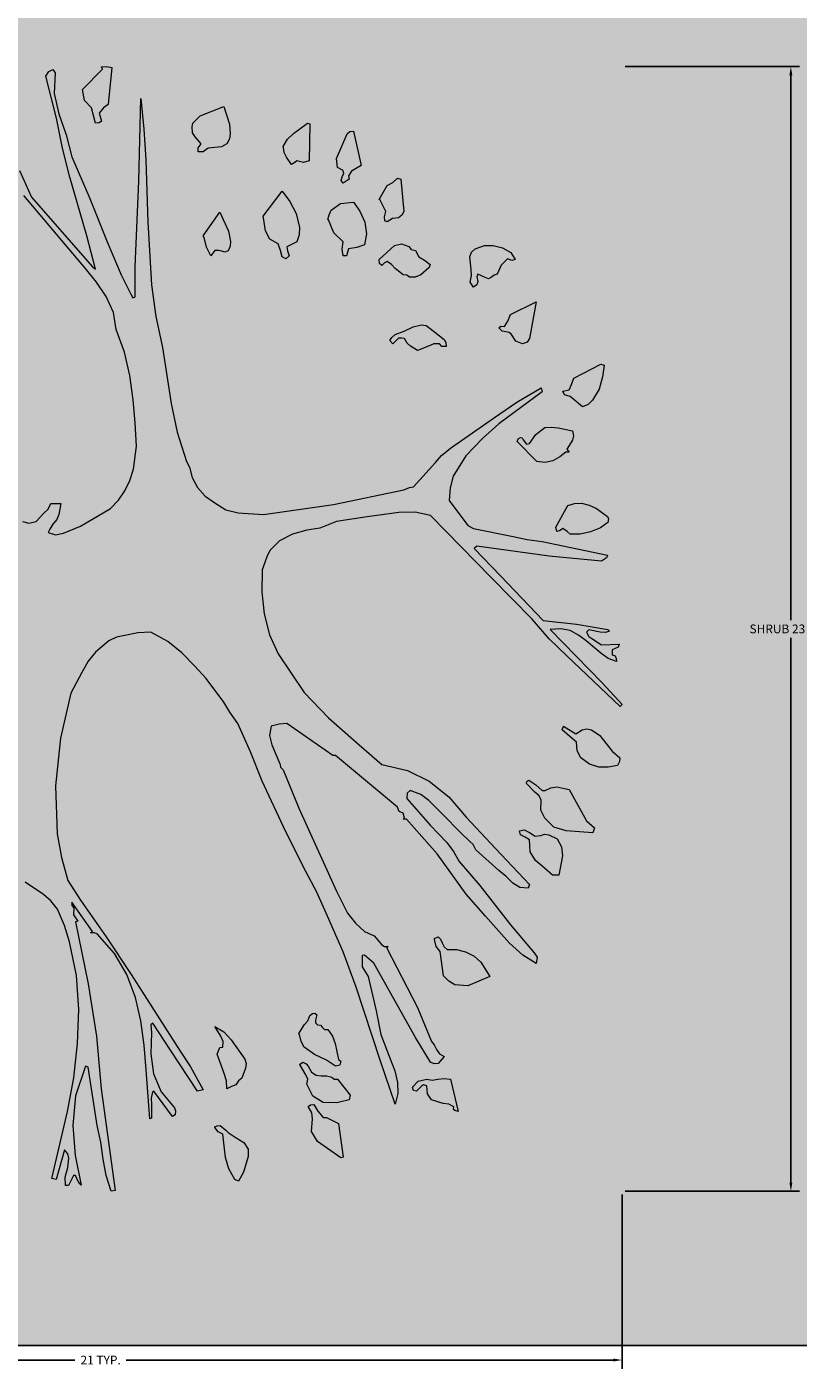
# Model space of a CAD drawing. Units: inches. Extents: x 84 to 1044, y -280 to 906.
# Tile 19 of 105: x 684 to 700, y -113 to -86. Entities that reach past the tile are written whole.
import ezdxf

# ---------------------------------------------------------------- set-up
doc = ezdxf.new("R2010")
doc.units = ezdxf.units.IN
for name, color, linetype, lineweight in [('A-ANNO-DIMS', 2, 'Continuous', 18), ('C-PROP', 7, 'Continuous', 25), ('L-PLNT', 114, 'Continuous', 15)]:
    doc.layers.add(name, color=color, linetype=linetype, lineweight=lineweight)
doc.layers.add('L-PLNT-PATT', color=9, linetype='Continuous', lineweight=9, true_color=0xafd9aa)
doc.styles.get("Standard").update_dxf_attribs({"font": 'arial.ttf'})
doc.dimstyles.get("Standard").update_dxf_attribs({"dimtxt": 0.18, "dimasz": 0.18, "dimexe": 0.18, "dimexo": 0.0625, "dimgap": 0.09, "dimtad": 0, "dimtih": 1, "dimtoh": 1, "dimdec": 4, "dimzin": 0, "dimdsep": 46, "dimtxsty": 'Standard', "dimcen": 0.09, "dimadec": 0, "dimazin": 0, "dimtfac": 1, "dimtdec": 4, "dimtofl": 0, "dimtmove": 0, "dimatfit": 3, "dimfxl": 1, "dimtolj": 1, "dimtzin": 0, "dimarcsym": 0})

# ---------------------------------------------------------------- blocks, each defined once
blk = doc.blocks.new('A$C37E508DF')
for p, q in [((0.6329, 1.5111), (0.6367, 1.5175)), ((0.6367, 1.5175), (0.6423, 1.5201)), ((0.6423, 1.5201), (0.6453, 1.5158)), ((0.6453, 1.5158), (0.644, 1.4879)), ((0.6826, 1.493), (0.7096, 1.5209)), ((0.7083, 1.5239), (0.7152, 1.5244)), ((0.7096, 1.5209), (0.7083, 1.5239)), ((0.7152, 1.5244), (0.7225, 1.5231)), ((0.7225, 1.5231), (0.7174, 1.4729)), ((0.6475, 1.4545), (0.6329, 1.5111)), ((0.644, 1.4879), (0.6505, 1.46)), ((0.6852, 1.4785), (0.6826, 1.493)), ((0.6946, 1.4682), (0.6852, 1.4785)), ((0.7589, 1.3691), (0.7615, 1.481)), ((0.7615, 1.481), (0.7658, 1.4395)), ((0.6505, 1.46), (0.6603, 1.4317)), ((0.6976, 1.4579), (0.6946, 1.4682)), ((0.7109, 1.4682), (0.7053, 1.4609)), ((0.7053, 1.4609), (0.7083, 1.4502)), ((0.7174, 1.4729), (0.7109, 1.4682)), ((0.8421, 1.4575), (0.8739, 1.4703)), ((0.8739, 1.4703), (0.882, 1.4463)), ((0.6552, 1.4137), (0.6475, 1.4545)), ((0.7002, 1.4476), (0.6976, 1.4579)), ((0.7049, 1.448), (0.7002, 1.4476)), ((0.7083, 1.4502), (0.7049, 1.448)), ((0.831, 1.4424), (0.8323, 1.4476)), ((0.8318, 1.4343), (0.831, 1.4424)), ((0.8323, 1.4476), (0.8357, 1.451)), ((0.8357, 1.451), (0.8421, 1.4575)), ((0.882, 1.4463), (0.8829, 1.433)), ((0.9686, 1.4334), (0.9875, 1.4476)), ((0.9875, 1.4476), (0.9905, 1.4467)), ((0.9905, 1.4467), (0.9896, 1.3966)), ((0.6603, 1.4317), (0.668, 1.4021)), ((0.7658, 1.4395), (0.7684, 1.3979)), ((0.8353, 1.4292), (0.8318, 1.4343)), ((0.8434, 1.4197), (0.8353, 1.4292)), ((0.8816, 1.4262), (0.8781, 1.4197)), ((0.8829, 1.433), (0.8816, 1.4262)), ((0.9545, 1.4159), (0.9605, 1.4257)), ((0.9605, 1.4257), (0.9686, 1.4334)), ((1.0269, 1.3996), (1.0411, 1.433)), ((1.0411, 1.433), (1.045, 1.4365)), ((1.045, 1.4365), (1.0497, 1.4369)), ((1.0497, 1.4369), (1.0604, 1.3901)), ((0.6655, 1.3743), (0.6552, 1.4137)), ((0.8391, 1.4141), (0.8434, 1.4197)), ((0.8395, 1.4086), (0.8391, 1.4141)), ((0.846, 1.4086), (0.8395, 1.4086)), ((0.8528, 1.4137), (0.846, 1.4086)), ((0.8619, 1.4146), (0.8528, 1.4137)), ((0.8709, 1.4154), (0.8619, 1.4146)), ((0.8781, 1.4197), (0.8709, 1.4154)), ((0.9549, 1.4146), (0.9545, 1.4159)), ((0.9558, 1.4077), (0.9549, 1.4146)), ((0.9592, 1.4017), (0.9558, 1.4077)), ((0.668, 1.4021), (0.6925, 1.3455)), ((0.7684, 1.3979), (0.771, 1.3134)), ((0.966, 1.3914), (0.9592, 1.4017)), ((0.9703, 1.3944), (0.966, 1.3914)), ((0.9733, 1.3966), (0.9703, 1.3944)), ((0.9819, 1.3944), (0.9733, 1.3966)), ((0.9896, 1.3966), (0.9819, 1.3944)), ((1.0282, 1.3876), (1.0269, 1.3996)), ((1.0359, 1.3833), (1.0282, 1.3876)), ((1.0604, 1.3901), (1.0471, 1.3824)), ((0.5969, 1.3833), (0.6132, 1.3472)), ((0.6882, 1.2949), (0.6655, 1.3743)), ((0.7538, 1.2529), (0.7589, 1.3691)), ((1.0334, 1.37), (1.0351, 1.376)), ((1.0359, 1.3661), (1.0334, 1.37)), ((1.0351, 1.376), (1.0368, 1.3794)), ((1.0368, 1.3794), (1.0359, 1.3833)), ((1.0441, 1.3717), (1.0359, 1.3661)), ((1.0471, 1.3824), (1.0432, 1.3764)), ((1.0432, 1.3764), (1.0441, 1.3717)), ((1.1033, 1.367), (1.1097, 1.373)), ((1.1097, 1.373), (1.114, 1.3717)), ((1.114, 1.3717), (1.1183, 1.328)), ((0.9274, 1.3215), (0.9532, 1.3554)), ((0.9532, 1.3554), (0.9635, 1.3413)), ((1.0848, 1.3443), (1.0955, 1.3631)), ((1.0955, 1.3631), (1.1033, 1.367)), ((0.6595, 1.2829), (0.6029, 1.3494)), ((0.6132, 1.3472), (0.6959, 1.2529)), ((0.6925, 1.3455), (0.7161, 1.2868)), ((0.9635, 1.3413), (0.9721, 1.325)), ((1.0197, 1.3297), (1.0321, 1.3387)), ((1.0321, 1.3387), (1.0497, 1.3404)), ((1.0497, 1.3404), (1.0587, 1.3284)), ((1.0861, 1.343), (1.0848, 1.3443)), ((1.0938, 1.328), (1.0861, 1.343)), ((0.846, 1.2949), (0.8687, 1.3271)), ((0.8687, 1.3271), (0.8803, 1.3014)), ((0.9279, 1.3194), (0.9274, 1.3215)), ((0.9305, 1.3018), (0.9279, 1.3194)), ((0.9721, 1.325), (0.9768, 1.3061)), ((1.0149, 1.3172), (1.0171, 1.3232)), ((1.0162, 1.3164), (1.0149, 1.3172)), ((1.0231, 1.2988), (1.0162, 1.3164)), ((1.0171, 1.3232), (1.0197, 1.3297)), ((1.0587, 1.3284), (1.0651, 1.3134)), ((1.0917, 1.3207), (1.0938, 1.328)), ((1.0925, 1.3151), (1.0917, 1.3207)), ((1.0955, 1.3138), (1.0925, 1.3151)), ((1.1028, 1.3185), (1.0955, 1.3138)), ((1.111, 1.3194), (1.1028, 1.3185)), ((1.1153, 1.3228), (1.111, 1.3194)), ((1.1183, 1.328), (1.1153, 1.3228)), ((0.771, 1.3134), (0.7761, 1.2285)), ((0.8803, 1.3014), (0.8833, 1.2872)), ((0.9365, 1.2902), (0.9305, 1.3018)), ((0.9763, 1.2962), (0.9733, 1.2868)), ((0.9768, 1.3061), (0.9763, 1.2962)), ((1.0359, 1.2868), (1.0231, 1.2988)), ((1.0677, 1.2975), (1.0647, 1.2829)), ((1.0651, 1.3134), (1.0677, 1.2975)), ((0.6865, 1.2508), (0.6595, 1.2829)), ((0.7002, 1.2495), (0.6882, 1.2949)), ((0.7161, 1.2868), (0.7349, 1.2422)), ((0.8473, 1.2924), (0.846, 1.2949)), ((0.8507, 1.2795), (0.8473, 1.2924)), ((0.8567, 1.2679), (0.8507, 1.2795)), ((0.8829, 1.2808), (0.8799, 1.2744)), ((0.8833, 1.2872), (0.8829, 1.2808)), ((0.9476, 1.2842), (0.9365, 1.2902)), ((0.951, 1.2748), (0.9476, 1.2842)), ((0.9733, 1.2868), (0.9596, 1.2799)), ((0.9596, 1.2799), (0.9605, 1.2744)), ((1.0347, 1.2769), (1.0359, 1.2868)), ((1.0432, 1.2774), (1.0402, 1.2679)), ((1.0544, 1.2791), (1.0432, 1.2774)), ((1.0647, 1.2829), (1.0544, 1.2791)), ((1.0848, 1.2628), (1.1054, 1.2817)), ((1.1054, 1.2817), (1.1148, 1.2842)), ((1.1148, 1.2842), (1.1247, 1.2804)), ((1.1247, 1.2804), (1.1281, 1.2765)), ((1.21, 1.2726), (1.2147, 1.2774)), ((1.2147, 1.2774), (1.2276, 1.2817)), ((1.2276, 1.2817), (1.2392, 1.2817)), ((1.2392, 1.2817), (1.2521, 1.2787)), ((1.2521, 1.2787), (1.2632, 1.2722)), ((0.8619, 1.2752), (0.8567, 1.2679)), ((0.867, 1.2752), (0.8619, 1.2752)), ((0.8713, 1.2739), (0.867, 1.2752)), ((0.8756, 1.2726), (0.8713, 1.2739)), ((0.8799, 1.2744), (0.8756, 1.2726)), ((0.9532, 1.2666), (0.951, 1.2748)), ((0.9583, 1.2636), (0.9532, 1.2666)), ((0.9626, 1.2679), (0.9583, 1.2636)), ((0.9605, 1.2744), (0.9626, 1.2679)), ((1.0359, 1.2679), (1.0347, 1.2769)), ((1.0402, 1.2679), (1.0359, 1.2679)), ((1.0852, 1.2576), (1.0848, 1.2628)), ((1.0955, 1.2602), (1.0921, 1.2585)), ((1.1015, 1.2559), (1.0955, 1.2602)), ((1.1281, 1.2765), (1.1341, 1.2752)), ((1.1341, 1.2752), (1.1384, 1.2666)), ((1.1384, 1.2666), (1.1461, 1.2619)), ((1.1461, 1.2619), (1.1539, 1.2559)), ((1.2075, 1.2666), (1.21, 1.2726)), ((1.2096, 1.2491), (1.2075, 1.2666)), ((1.2585, 1.2636), (1.2503, 1.2551)), ((1.2645, 1.2615), (1.2585, 1.2636)), ((1.2632, 1.2722), (1.2692, 1.2628)), ((1.2692, 1.2628), (1.2645, 1.2615)), ((0.7015, 1.2323), (0.6865, 1.2508)), ((0.6959, 1.2529), (0.7002, 1.2495)), ((0.7349, 1.2422), (0.7482, 1.216)), ((0.7538, 1.2122), (0.7538, 1.2529)), ((1.0883, 1.2546), (1.0852, 1.2576)), ((1.0921, 1.2585), (1.0883, 1.2546)), ((1.1063, 1.2508), (1.1015, 1.2559)), ((1.117, 1.2422), (1.1063, 1.2508)), ((1.1221, 1.2418), (1.117, 1.2422)), ((1.126, 1.2388), (1.1221, 1.2418)), ((1.141, 1.2422), (1.1337, 1.2388)), ((1.1526, 1.2521), (1.141, 1.2422)), ((1.1539, 1.2559), (1.1526, 1.2521)), ((1.2079, 1.2323), (1.21, 1.2409)), ((1.21, 1.2409), (1.2096, 1.2491)), ((1.2186, 1.2431), (1.2173, 1.2392)), ((1.2285, 1.2383), (1.2186, 1.2431)), ((1.2405, 1.2418), (1.2371, 1.2388)), ((1.2448, 1.2431), (1.2405, 1.2418)), ((1.2503, 1.2551), (1.2448, 1.2431)), ((0.7148, 1.2126), (0.7015, 1.2323)), ((0.7761, 1.2285), (0.7821, 1.1856)), ((1.1337, 1.2388), (1.126, 1.2388)), ((1.2126, 1.2251), (1.2079, 1.2323)), ((1.2169, 1.2285), (1.2126, 1.2251)), ((1.2186, 1.2332), (1.2169, 1.2285)), ((1.2173, 1.2392), (1.2186, 1.2332)), ((1.2328, 1.2366), (1.2285, 1.2383)), ((1.2371, 1.2388), (1.2328, 1.2366)), ((0.7246, 1.1908), (0.7148, 1.2126)), ((0.7482, 1.216), (0.7508, 1.2109)), ((0.7508, 1.2109), (0.7538, 1.2122)), ((1.2628, 1.1882), (1.2975, 1.2053)), ((1.2975, 1.2053), (1.2885, 1.1556)), ((0.7281, 1.168), (0.7246, 1.1908)), ((1.2589, 1.1792), (1.2628, 1.1882)), ((0.7396, 1.1371), (0.7281, 1.168)), ((0.7821, 1.1856), (0.7911, 1.1436)), ((1.1187, 1.1655), (1.1307, 1.1714)), ((1.1307, 1.1714), (1.1423, 1.1744)), ((1.1423, 1.1744), (1.1483, 1.1732)), ((1.1483, 1.1732), (1.1539, 1.1693)), ((1.1539, 1.1693), (1.1727, 1.1543)), ((1.2469, 1.1702), (1.2495, 1.1723)), ((1.2478, 1.1693), (1.2469, 1.1702)), ((1.2516, 1.1659), (1.2478, 1.1693)), ((1.2495, 1.1723), (1.2546, 1.1719)), ((1.2546, 1.1719), (1.2589, 1.1792)), ((1.099, 1.153), (1.102, 1.1573)), ((1.1033, 1.1487), (1.099, 1.153)), ((1.102, 1.1573), (1.1063, 1.1612)), ((1.111, 1.156), (1.1033, 1.1487)), ((1.1063, 1.1612), (1.1187, 1.1655)), ((1.1153, 1.1564), (1.111, 1.156)), ((1.1191, 1.1556), (1.1153, 1.1564)), ((1.1226, 1.1492), (1.1191, 1.1556)), ((1.1727, 1.1543), (1.1749, 1.1504)), ((1.1749, 1.1504), (1.1757, 1.1449)), ((1.2563, 1.1646), (1.2516, 1.1659)), ((1.2611, 1.1637), (1.2563, 1.1646)), ((1.2641, 1.1612), (1.2611, 1.1637)), ((1.2701, 1.1522), (1.2641, 1.1612)), ((1.2791, 1.1487), (1.2701, 1.1522)), ((1.2851, 1.1509), (1.2791, 1.1487)), ((1.2885, 1.1556), (1.2851, 1.1509)), ((0.7469, 1.1054), (0.7396, 1.1371)), ((0.7911, 1.1436), (0.8027, 1.0677)), ((1.1273, 1.1453), (1.1226, 1.1492)), ((1.1367, 1.1393), (1.1273, 1.1453)), ((1.1517, 1.1453), (1.1367, 1.1393)), ((1.1586, 1.1483), (1.1517, 1.1453)), ((1.1663, 1.1487), (1.1586, 1.1483)), ((1.1697, 1.1449), (1.1663, 1.1487)), ((1.1757, 1.1449), (1.1697, 1.1449)), ((1.3485, 1.102), (1.385, 1.1209)), ((1.385, 1.1209), (1.3897, 1.1196)), ((1.3897, 1.1196), (1.3875, 1.1037)), ((0.7512, 1.0728), (0.7469, 1.1054)), ((1.3455, 1.0934), (1.3485, 1.102)), ((1.3875, 1.1037), (1.3828, 1.087)), ((1.3057, 1.0835), (1.2469, 1.0402)), ((1.2713, 1.0694), (1.3044, 1.0887)), ((1.3044, 1.0887), (1.3057, 1.0835)), ((1.3335, 1.0844), (1.3421, 1.0861)), ((1.3361, 1.0793), (1.3335, 1.0844)), ((1.3434, 1.0771), (1.3361, 1.0793)), ((1.3421, 1.0861), (1.3455, 1.0934)), ((1.349, 1.0728), (1.3434, 1.0771)), ((1.3828, 1.087), (1.3738, 1.072)), ((0.7538, 1.0415), (0.7512, 1.0728)), ((0.8027, 1.0677), (0.8108, 1.0287)), ((1.2409, 1.0488), (1.2713, 1.0694)), ((1.3605, 1.063), (1.349, 1.0728)), ((1.3678, 1.0664), (1.3605, 1.063)), ((1.3738, 1.072), (1.3678, 1.0664)), ((0.7559, 1.0098), (0.7538, 1.0415)), ((1.1813, 1.0072), (1.2409, 1.0488)), ((1.2469, 1.0402), (1.2246, 1.0201)), ((0.8108, 1.0287), (0.8233, 0.9892)), ((1.2731, 1.0197), (1.2761, 1.0218)), ((1.2761, 1.0218), (1.2786, 1.0209)), ((1.2885, 1.0136), (1.2971, 1.0257)), ((1.2971, 1.0257), (1.3091, 1.0351)), ((1.3091, 1.0351), (1.3185, 1.0355)), ((1.3185, 1.0355), (1.3275, 1.0347)), ((1.3275, 1.0347), (1.3468, 1.0308)), ((1.3468, 1.0308), (1.3481, 1.0239)), ((1.3481, 1.0239), (1.3468, 1.018)), ((0.7516, 0.9785), (0.7559, 1.0098)), ((1.1693, 0.9974), (1.1813, 1.0072)), ((1.2246, 1.0201), (1.2023, 0.9969)), ((1.2718, 1.0162), (1.2731, 1.0197)), ((1.2984, 0.9892), (1.2718, 1.0162)), ((1.2786, 1.0209), (1.2799, 1.0184)), ((1.2799, 1.0184), (1.2842, 1.0124)), ((1.2842, 1.0124), (1.2885, 1.0136)), ((1.3468, 1.018), (1.3391, 1.0059)), ((1.3391, 1.0059), (1.3421, 1.0016)), ((0.8233, 0.9892), (0.8275, 0.9815)), ((1.1311, 0.9549), (1.1612, 0.9879)), ((1.1612, 0.9879), (1.1693, 0.9974)), ((1.2023, 0.9969), (1.1852, 0.9691)), ((1.3095, 0.9875), (1.2984, 0.9892)), ((1.3202, 0.9901), (1.3095, 0.9875)), ((1.3297, 0.9952), (1.3202, 0.9901)), ((1.3378, 1.0016), (1.3297, 0.9952)), ((1.3421, 1.0016), (1.3378, 1.0016)), ((0.7469, 0.9635), (0.7516, 0.9785)), ((0.8275, 0.9815), (0.8314, 0.9673)), ((0.8314, 0.9673), (0.8383, 0.954)), ((1.1852, 0.9691), (1.1809, 0.9532)), ((0.7315, 0.9365), (0.7401, 0.9493)), ((0.7401, 0.9493), (0.7469, 0.9635)), ((0.8383, 0.954), (0.8486, 0.942)), ((1.0227, 0.9309), (1.1183, 0.9506)), ((1.1183, 0.9506), (1.1256, 0.954)), ((1.1256, 0.954), (1.1311, 0.9549)), ((1.1809, 0.9532), (1.1796, 0.936)), ((0.6359, 0.9245), (0.6397, 0.9322)), ((0.6397, 0.9322), (0.653, 0.9322)), ((0.653, 0.9322), (0.6505, 0.9172)), ((0.7203, 0.9253), (0.7315, 0.9365)), ((0.8486, 0.942), (0.8619, 0.933)), ((0.8619, 0.933), (0.8769, 0.9236)), ((0.9279, 0.9172), (1.0227, 0.9309)), ((1.1796, 0.936), (1.2049, 0.9022)), ((1.3404, 0.9292), (1.3494, 0.9322)), ((1.3494, 0.9322), (1.3592, 0.9326)), ((1.3592, 0.9326), (1.3695, 0.93)), ((0.6196, 0.9077), (0.6303, 0.9189)), ((0.6303, 0.9189), (0.6359, 0.9245)), ((0.6505, 0.9172), (0.6479, 0.9103)), ((0.6796, 0.9013), (0.7203, 0.9253)), ((0.8769, 0.9236), (0.8936, 0.9193)), ((0.8936, 0.9193), (0.9279, 0.9172)), ((1.0685, 0.9142), (1.0269, 0.9077)), ((1.1114, 0.9198), (1.0685, 0.9142)), ((1.1333, 0.9202), (1.1114, 0.9198)), ((1.1543, 0.9159), (1.1333, 0.9202)), ((1.2371, 0.8314), (1.1543, 0.9159)), ((1.3241, 0.9), (1.3404, 0.9292)), ((1.3695, 0.93), (1.3794, 0.9253)), ((1.3794, 0.9253), (1.394, 0.9146)), ((1.394, 0.9146), (1.3957, 0.9112)), ((0.6011, 0.9077), (0.6097, 0.9056)), ((0.6097, 0.9056), (0.6196, 0.9077)), ((0.6384, 0.8974), (0.6359, 0.8927)), ((0.6423, 0.9039), (0.6384, 0.8974)), ((0.6479, 0.9103), (0.6423, 0.9039)), ((0.6569, 0.8919), (0.6796, 0.9013)), ((0.9866, 0.8962), (0.9673, 0.8906)), ((1.0042, 0.8987), (0.9866, 0.8962)), ((1.0269, 0.9077), (1.0042, 0.8987)), ((1.2049, 0.9022), (1.2126, 0.8983)), ((1.2126, 0.8983), (1.2662, 0.8876)), ((1.3254, 0.8944), (1.3241, 0.9)), ((1.3301, 0.8957), (1.3254, 0.8944)), ((1.3335, 0.8983), (1.3301, 0.8957)), ((1.3395, 0.8944), (1.3335, 0.8983)), ((1.3434, 0.8906), (1.3395, 0.8944)), ((1.3846, 0.8992), (1.3713, 0.8936)), ((1.3948, 0.9065), (1.3846, 0.8992)), ((1.3957, 0.9112), (1.3948, 0.9065)), ((0.6359, 0.8927), (0.6457, 0.8897)), ((0.6457, 0.8897), (0.6569, 0.8919)), ((0.9498, 0.8816), (0.9369, 0.8687)), ((0.9673, 0.8906), (0.9498, 0.8816)), ((1.2662, 0.8876), (1.2855, 0.8833)), ((1.2855, 0.8833), (1.3057, 0.8807)), ((1.3057, 0.8807), (1.394, 0.8623)), ((1.3571, 0.8906), (1.3434, 0.8906)), ((1.3713, 0.8936), (1.3571, 0.8906)), ((0.933, 0.861), (0.9296, 0.852)), ((0.9369, 0.8687), (0.933, 0.861)), ((1.2169, 0.8743), (1.2135, 0.8713)), ((1.2135, 0.8713), (1.2491, 0.834)), ((1.3151, 0.8606), (1.2169, 0.8743)), ((1.3863, 0.8541), (1.3151, 0.8606)), ((1.3927, 0.8584), (1.3863, 0.8541)), ((1.394, 0.8623), (1.3927, 0.8584)), ((0.9262, 0.8421), (0.9257, 0.8121)), ((0.9296, 0.852), (0.9262, 0.8421)), ((1.2919, 0.7752), (1.2371, 0.8314)), ((1.2491, 0.834), (1.3069, 0.7735)), ((0.9257, 0.8121), (0.9287, 0.7825)), ((0.9287, 0.7825), (0.936, 0.7542)), ((1.3151, 0.7487), (1.2919, 0.7752)), ((1.3069, 0.7735), (1.352, 0.7684)), ((1.352, 0.7684), (1.3948, 0.7615)), ((0.7285, 0.7512), (0.7182, 0.7461)), ((0.7401, 0.7534), (0.7285, 0.7512)), ((0.7577, 0.7568), (0.7401, 0.7534)), ((0.7752, 0.7577), (0.7577, 0.7568)), ((0.798, 0.7452), (0.7752, 0.7577)), ((0.936, 0.7542), (0.9476, 0.7285)), ((1.3391, 0.7255), (1.3151, 0.7487)), ((1.3309, 0.7624), (1.3164, 0.7615)), ((1.3164, 0.7615), (1.3871, 0.6891)), ((1.3434, 0.7598), (1.3309, 0.7624)), ((1.355, 0.7538), (1.3434, 0.7598)), ((1.3653, 0.7461), (1.355, 0.7538)), ((1.3687, 0.7607), (1.3657, 0.7577)), ((1.3657, 0.7577), (1.3691, 0.7521)), ((1.3841, 0.7577), (1.3687, 0.7607)), ((1.3691, 0.7521), (1.3743, 0.7482)), ((1.3743, 0.7482), (1.3863, 0.7405)), ((1.3914, 0.7572), (1.3841, 0.7577)), ((1.397, 0.759), (1.3914, 0.7572)), ((1.3948, 0.7615), (1.397, 0.759)), ((0.7002, 0.7307), (0.6903, 0.7186)), ((0.7182, 0.7461), (0.7002, 0.7307)), ((0.8173, 0.7298), (0.798, 0.7452)), ((0.8344, 0.7122), (0.8173, 0.7298)), ((1.3854, 0.7294), (1.3653, 0.7461)), ((1.3863, 0.7405), (1.4099, 0.7414)), ((1.4086, 0.7375), (1.4004, 0.7337)), ((1.4004, 0.7337), (1.4004, 0.7272)), ((1.4099, 0.7414), (1.4086, 0.7375)), ((0.6903, 0.7186), (0.6818, 0.7032)), ((0.8503, 0.6951), (0.8344, 0.7122)), ((0.9476, 0.7285), (0.9828, 0.6762)), ((1.4116, 0.6569), (1.3391, 0.7255)), ((1.3953, 0.7221), (1.3854, 0.7294)), ((1.4064, 0.7178), (1.3953, 0.7221)), ((1.4004, 0.7272), (1.4047, 0.7255)), ((1.4047, 0.7255), (1.406, 0.7221)), ((1.406, 0.7221), (1.4064, 0.7178)), ((0.6818, 0.7032), (0.6667, 0.6749)), ((0.8739, 0.6629), (0.8503, 0.6951)), ((0.9828, 0.6762), (1.0162, 0.6415)), ((1.3871, 0.6891), (1.4141, 0.6599)), ((0.6667, 0.6749), (0.6526, 0.614)), ((0.8824, 0.6492), (0.8739, 0.6629)), ((1.4141, 0.6599), (1.4116, 0.6569)), ((0.8932, 0.6342), (0.8824, 0.6492)), ((1.0162, 0.6415), (1.0574, 0.605)), ((0.9103, 0.5956), (0.8932, 0.6342)), ((0.9382, 0.6303), (0.936, 0.6179)), ((0.9493, 0.6333), (0.9382, 0.6303)), ((0.9596, 0.6342), (0.9493, 0.6333)), ((1.0218, 0.5904), (0.9596, 0.6342)), ((1.3327, 0.6252), (1.3348, 0.6303)), ((1.343, 0.6162), (1.3327, 0.6252)), ((1.3348, 0.6303), (1.3511, 0.62)), ((1.3511, 0.62), (1.3601, 0.6256)), ((1.3601, 0.6256), (1.3661, 0.6269)), ((1.3661, 0.6269), (1.3725, 0.6252)), ((1.3725, 0.6252), (1.3837, 0.6175)), ((0.6526, 0.614), (0.6457, 0.5497)), ((0.936, 0.6179), (0.939, 0.605)), ((0.939, 0.605), (0.9506, 0.5784)), ((1.0574, 0.605), (1.0883, 0.5784)), ((1.352, 0.6089), (1.343, 0.6162)), ((1.3533, 0.5969), (1.352, 0.6089)), ((1.3837, 0.6175), (1.3918, 0.6072)), ((1.3918, 0.6072), (1.4004, 0.5964)), ((0.9262, 0.5557), (0.9103, 0.5956)), ((1.0256, 0.5904), (1.0218, 0.5904)), ((1.1097, 0.5205), (1.0256, 0.5904)), ((1.358, 0.5874), (1.3533, 0.5969)), ((1.37, 0.5789), (1.358, 0.5874)), ((1.4004, 0.5964), (1.4111, 0.5874)), ((1.4111, 0.5874), (1.4103, 0.5823)), ((0.9506, 0.5784), (0.951, 0.5746)), ((0.951, 0.5746), (0.9545, 0.5711)), ((0.9545, 0.5711), (0.9759, 0.5193)), ((1.0883, 0.5784), (1.123, 0.5703)), ((1.123, 0.5703), (1.1526, 0.5557)), ((1.3824, 0.575), (1.37, 0.5789)), ((1.3953, 0.5746), (1.3824, 0.575)), ((1.4077, 0.5771), (1.3953, 0.5746)), ((1.4103, 0.5823), (1.4077, 0.5771)), ((0.6457, 0.5497), (0.6483, 0.4845)), ((0.9583, 0.4871), (0.9262, 0.5557)), ((1.1526, 0.5557), (1.1792, 0.5347)), ((1.2842, 0.554), (1.2855, 0.5557)), ((1.2842, 0.5527), (1.2842, 0.554)), ((1.2958, 0.5407), (1.2842, 0.5527)), ((1.2855, 0.5557), (1.2876, 0.557)), ((1.2876, 0.557), (1.2971, 0.551)), ((1.2971, 0.551), (1.3057, 0.5433)), ((1.3172, 0.5467), (1.3254, 0.548)), ((1.3254, 0.548), (1.3421, 0.5446)), ((1.1226, 0.5394), (1.1221, 0.5325)), ((1.1221, 0.5325), (1.1539, 0.4961)), ((1.1268, 0.5433), (1.1226, 0.5394)), ((1.141, 0.5377), (1.1268, 0.5433)), ((1.1521, 0.5296), (1.141, 0.5377)), ((1.1706, 0.5111), (1.1521, 0.5296)), ((1.1792, 0.5347), (1.2027, 0.5072)), ((1.3014, 0.536), (1.2958, 0.5407)), ((1.3044, 0.53), (1.3014, 0.536)), ((1.3039, 0.5167), (1.3044, 0.53)), ((1.3057, 0.5433), (1.3099, 0.5433)), ((1.3099, 0.5433), (1.3172, 0.5467)), ((1.3421, 0.5446), (1.3657, 0.5021)), ((0.9759, 0.5193), (1.0269, 0.4069)), ((1.1118, 0.5145), (1.1097, 0.5205)), ((1.117, 0.5124), (1.1118, 0.5145)), ((1.1191, 0.5055), (1.117, 0.5124)), ((1.1955, 0.4858), (1.1706, 0.5111)), ((1.3091, 0.5055), (1.3039, 0.5167)), ((1.117, 0.5042), (1.1191, 0.5055)), ((1.1217, 0.5042), (1.117, 0.5042)), ((1.1633, 0.4575), (1.1217, 0.5042)), ((1.1539, 0.4961), (1.1762, 0.4729)), ((1.2027, 0.5072), (1.2426, 0.4644)), ((1.3215, 0.4935), (1.3091, 0.5055)), ((1.3382, 0.4884), (1.3215, 0.4935)), ((1.3657, 0.5021), (1.3764, 0.4927)), ((1.3764, 0.4927), (1.3743, 0.4858)), ((0.6483, 0.4845), (0.6539, 0.4524)), ((0.9853, 0.4335), (0.9583, 0.4871)), ((1.207, 0.4747), (1.1955, 0.4858)), ((1.2122, 0.47), (1.207, 0.4747)), ((1.2748, 0.4884), (1.2812, 0.4897)), ((1.2761, 0.4832), (1.2748, 0.4884)), ((1.2825, 0.4798), (1.2761, 0.4832)), ((1.2812, 0.4897), (1.2885, 0.4862)), ((1.2885, 0.4764), (1.2825, 0.4798)), ((1.2885, 0.4862), (1.2962, 0.4815)), ((1.2894, 0.4601), (1.2885, 0.4764)), ((1.2962, 0.4815), (1.3039, 0.482)), ((1.3039, 0.482), (1.3087, 0.4841)), ((1.3087, 0.4841), (1.3147, 0.4832)), ((1.3147, 0.4832), (1.3258, 0.4777)), ((1.3258, 0.4777), (1.3318, 0.4669)), ((1.3743, 0.4858), (1.3382, 0.4884)), ((1.2027, 0.4026), (1.1633, 0.4575)), ((1.1762, 0.4729), (1.1856, 0.4605)), ((1.1856, 0.4605), (1.1933, 0.4468)), ((1.2156, 0.4627), (1.2122, 0.47)), ((1.2469, 0.4348), (1.2156, 0.4627)), ((1.2426, 0.4644), (1.2885, 0.4159)), ((1.2967, 0.4485), (1.2894, 0.4601)), ((1.3318, 0.4669), (1.3331, 0.4545)), ((0.6539, 0.4524), (0.6625, 0.4211)), ((1.1933, 0.4468), (1.2212, 0.4146)), ((1.3082, 0.4386), (1.2967, 0.4485)), ((1.3198, 0.4284), (1.3082, 0.4386)), ((1.3331, 0.4545), (1.3284, 0.4284)), ((0.6625, 0.4211), (0.6796, 0.3945)), ((1.0003, 0.4052), (0.9853, 0.4335)), ((1.2568, 0.4266), (1.2469, 0.4348)), ((1.2658, 0.4176), (1.2568, 0.4266)), ((1.3284, 0.4284), (1.3198, 0.4284)), ((0.6295, 0.4022), (0.6046, 0.4189)), ((0.6397, 0.3936), (0.6295, 0.4022)), ((1.0145, 0.373), (1.0003, 0.4052)), ((1.0269, 0.4069), (1.0419, 0.3769)), ((1.2289, 0.373), (1.2027, 0.4026)), ((1.2212, 0.4146), (1.2628, 0.361)), ((1.2752, 0.4116), (1.2658, 0.4176)), ((1.2868, 0.4108), (1.2752, 0.4116)), ((1.2885, 0.4159), (1.2868, 0.4108)), ((0.6487, 0.3825), (0.6397, 0.3936)), ((0.6959, 0.352), (0.668, 0.3919)), ((0.668, 0.3919), (0.668, 0.3872)), ((0.668, 0.3872), (0.6706, 0.3842)), ((0.6706, 0.3842), (0.6702, 0.3748)), ((0.6796, 0.3945), (0.7148, 0.3447)), ((0.6582, 0.3602), (0.6487, 0.3825)), ((0.6702, 0.3748), (0.6762, 0.3662)), ((0.6762, 0.3662), (0.6732, 0.3653)), ((0.6732, 0.3653), (0.6903, 0.2813)), ((1.0359, 0.3246), (1.0145, 0.373)), ((1.0419, 0.3769), (1.0527, 0.3632)), ((1.2615, 0.3362), (1.2289, 0.373)), ((0.665, 0.3379), (0.6582, 0.3602)), ((0.6933, 0.3503), (0.6959, 0.352)), ((0.6985, 0.3503), (0.6933, 0.3503)), ((0.7023, 0.349), (0.6985, 0.3503)), ((0.7259, 0.3224), (0.7023, 0.349)), ((1.0527, 0.3632), (1.0647, 0.352)), ((1.0647, 0.352), (1.078, 0.346)), ((1.2628, 0.361), (1.2949, 0.3233)), ((0.6745, 0.2924), (0.665, 0.3379)), ((0.7148, 0.3447), (0.7487, 0.2937)), ((1.078, 0.346), (1.0883, 0.334)), ((1.0883, 0.334), (1.0921, 0.3319)), ((1.0921, 0.3319), (1.0968, 0.3319)), ((1.0968, 0.3319), (1.0947, 0.3306)), ((1.0947, 0.3306), (1.1367, 0.2491)), ((1.1599, 0.3426), (1.1646, 0.3447)), ((1.1599, 0.3413), (1.1599, 0.3426)), ((1.162, 0.3319), (1.1599, 0.3413)), ((1.1676, 0.325), (1.162, 0.3319)), ((1.1646, 0.3447), (1.168, 0.3417)), ((1.168, 0.3417), (1.1702, 0.3366)), ((1.1702, 0.3366), (1.1727, 0.3314)), ((1.1727, 0.3314), (1.177, 0.3276)), ((1.2795, 0.3199), (1.2615, 0.3362)), ((0.7427, 0.2937), (0.7259, 0.3224)), ((1.0535, 0.2766), (1.0359, 0.3246)), ((1.0647, 0.3199), (1.0617, 0.3194)), ((1.0617, 0.3194), (1.0617, 0.304)), ((1.0711, 0.3147), (1.0647, 0.3199)), ((1.0775, 0.3092), (1.0711, 0.3147)), ((1.1719, 0.292), (1.1676, 0.325)), ((1.177, 0.3276), (1.1895, 0.3276)), ((1.1895, 0.3276), (1.2019, 0.3246)), ((1.2019, 0.3246), (1.2135, 0.3186)), ((1.2135, 0.3186), (1.2225, 0.3104)), ((1.2225, 0.3104), (1.2349, 0.2911)), ((1.2975, 0.3087), (1.2795, 0.3199)), ((1.2949, 0.3233), (1.2988, 0.3173)), ((1.2988, 0.3173), (1.2975, 0.3087)), ((0.6775, 0.2465), (0.6745, 0.2924)), ((0.7542, 0.2628), (0.7427, 0.2937)), ((0.7487, 0.2937), (0.8151, 0.1899)), ((1.0617, 0.304), (1.0698, 0.2911)), ((1.1341, 0.2084), (1.0775, 0.3092)), ((1.1792, 0.2847), (1.1719, 0.292)), ((0.6903, 0.2813), (0.7015, 0.2101)), ((1.0861, 0.1775), (1.0535, 0.2766)), ((1.0698, 0.2911), (1.0805, 0.2448)), ((1.1873, 0.28), (1.1792, 0.2847)), ((1.2049, 0.2783), (1.1873, 0.28)), ((1.2349, 0.2911), (1.2049, 0.2783)), ((0.7615, 0.2311), (0.7542, 0.2628)), ((0.6758, 0.2002), (0.6775, 0.2465)), ((0.9879, 0.2311), (0.9905, 0.2384)), ((0.9905, 0.2384), (0.9943, 0.241)), ((0.9943, 0.241), (0.9973, 0.2414)), ((0.9973, 0.2414), (1.0003, 0.2393)), ((1.0003, 0.2393), (0.9986, 0.232)), ((1.0805, 0.2448), (1.087, 0.2127)), ((1.1367, 0.2491), (1.1556, 0.2032)), ((0.7662, 0.1981), (0.7615, 0.2311)), ((0.7778, 0.2277), (0.7752, 0.2255)), ((0.7752, 0.2255), (0.7761, 0.2152)), ((0.8018, 0.1912), (0.7778, 0.2277)), ((0.8619, 0.2234), (0.8739, 0.2161)), ((0.87, 0.2101), (0.8619, 0.2234)), ((0.9759, 0.214), (0.9836, 0.226)), ((0.9836, 0.226), (0.9879, 0.2311)), ((0.9986, 0.232), (0.9986, 0.2281)), ((0.9986, 0.2281), (1.0012, 0.2255)), ((1.0012, 0.2255), (1.0051, 0.2251)), ((1.0051, 0.2251), (1.0076, 0.2225)), ((1.0076, 0.2225), (1.0106, 0.2195)), ((1.0106, 0.2195), (1.0149, 0.2191)), ((1.0149, 0.2191), (1.0214, 0.2101)), ((0.7015, 0.2101), (0.7079, 0.1389)), ((0.7761, 0.2152), (0.7752, 0.1861)), ((0.8734, 0.2032), (0.87, 0.2101)), ((0.8726, 0.1955), (0.8734, 0.2032)), ((0.8739, 0.2161), (0.8841, 0.2054)), ((0.8841, 0.2054), (0.9026, 0.1792)), ((0.9768, 0.2127), (0.9759, 0.214)), ((0.9789, 0.2028), (0.9768, 0.2127)), ((0.9832, 0.1955), (0.9789, 0.2028)), ((1.0214, 0.2101), (1.0252, 0.2002)), ((1.087, 0.2127), (1.0998, 0.1797)), ((1.1543, 0.1749), (1.1341, 0.2084)), ((1.1556, 0.2032), (1.1594, 0.1985)), ((0.6706, 0.1539), (0.6758, 0.2002)), ((0.7688, 0.1646), (0.7662, 0.1981)), ((0.7752, 0.1861), (0.7787, 0.1591)), ((0.8383, 0.1359), (0.8018, 0.1912)), ((0.8151, 0.1899), (0.8288, 0.1685)), ((0.8649, 0.1857), (0.8687, 0.1947)), ((0.8743, 0.1608), (0.8649, 0.1857)), ((0.8687, 0.1947), (0.8726, 0.1955)), ((0.9969, 0.1852), (0.9832, 0.1955)), ((1.0132, 0.1779), (0.9969, 0.1852)), ((1.0252, 0.2002), (1.0295, 0.1788)), ((1.1594, 0.1985), (1.1624, 0.1921)), ((1.1624, 0.1921), (1.1663, 0.1861)), ((1.1727, 0.1827), (1.1646, 0.1732)), ((1.1663, 0.1861), (1.1727, 0.1827)), ((0.6865, 0.1698), (0.6732, 0.1295)), ((0.6903, 0.1681), (0.6865, 0.1698)), ((0.7023, 0.0892), (0.6903, 0.1681)), ((0.774, 0.0982), (0.7688, 0.1646)), ((0.8288, 0.1685), (0.846, 0.1376)), ((0.9035, 0.1668), (0.8983, 0.1535)), ((0.9026, 0.1792), (0.9043, 0.1732)), ((0.9043, 0.1732), (0.9035, 0.1668)), ((0.9768, 0.1719), (0.9811, 0.1749)), ((0.9776, 0.1711), (0.9768, 0.1719)), ((0.9853, 0.1578), (0.9776, 0.1711)), ((0.9811, 0.1749), (0.9858, 0.1728)), ((0.9858, 0.1728), (0.9884, 0.1694)), ((0.9884, 0.1694), (0.9931, 0.1616)), ((1.0256, 0.1698), (1.0132, 0.1779)), ((1.0312, 0.1711), (1.0256, 0.1698)), ((1.0295, 0.1788), (1.0325, 0.1762)), ((1.0325, 0.1762), (1.0312, 0.1711)), ((1.1063, 0.1183), (1.0861, 0.1775)), ((1.0998, 0.1797), (1.1058, 0.1634)), ((1.1594, 0.1728), (1.1543, 0.1749)), ((1.1646, 0.1732), (1.1594, 0.1728)), ((0.662, 0.108), (0.6706, 0.1539)), ((0.7787, 0.1591), (0.789, 0.1346)), ((0.8777, 0.1496), (0.8743, 0.1608)), ((0.8781, 0.1389), (0.8777, 0.1496)), ((0.894, 0.1496), (0.8902, 0.1441)), ((0.8983, 0.1535), (0.894, 0.1496)), ((0.9879, 0.1518), (0.9853, 0.1578)), ((0.9866, 0.1453), (0.9879, 0.1518)), ((0.9931, 0.1616), (0.9991, 0.1574)), ((0.9991, 0.1574), (1.0059, 0.1565)), ((1.0059, 0.1565), (1.0132, 0.1565)), ((1.0132, 0.1565), (1.0205, 0.1548)), ((1.0205, 0.1548), (1.0235, 0.1522)), ((1.0235, 0.1522), (1.0282, 0.1518)), ((1.0282, 0.1518), (1.0454, 0.1303)), ((1.1058, 0.1634), (1.1097, 0.1475)), ((1.1097, 0.1475), (1.1101, 0.1325)), ((1.1298, 0.1411), (1.1376, 0.1492)), ((1.1376, 0.1492), (1.1491, 0.1518)), ((1.1491, 0.1518), (1.1564, 0.1505)), ((1.1564, 0.1505), (1.1642, 0.1518)), ((1.1642, 0.1518), (1.1727, 0.1531)), ((1.1727, 0.1531), (1.1813, 0.1518)), ((1.1813, 0.1518), (1.192, 0.108)), ((0.6732, 0.1295), (0.6693, 0.0892)), ((0.7079, 0.1389), (0.7268, 0.0013)), ((0.7774, 0.1346), (0.7757, 0.1261)), ((0.7791, 0.1359), (0.7774, 0.1346)), ((0.8044, 0.1012), (0.7791, 0.1359)), ((0.789, 0.1346), (0.8074, 0.1132)), ((0.846, 0.1376), (0.8383, 0.1359)), ((0.8846, 0.1419), (0.8781, 0.1389)), ((0.8902, 0.1441), (0.8846, 0.1419)), ((0.9948, 0.1291), (0.9866, 0.1453)), ((1.0089, 0.1205), (0.9948, 0.1291)), ((1.0454, 0.1303), (1.0441, 0.1239)), ((1.1101, 0.1325), (1.1063, 0.1183)), ((1.1311, 0.1364), (1.1298, 0.1411)), ((1.1354, 0.1359), (1.1311, 0.1364)), ((1.1384, 0.1389), (1.1354, 0.1359)), ((1.1423, 0.1423), (1.1384, 0.1389)), ((1.1449, 0.1441), (1.1423, 0.1423)), ((1.1491, 0.1428), (1.1449, 0.1441)), ((1.1504, 0.132), (1.1491, 0.1428)), ((1.1556, 0.1239), (1.1504, 0.132)), ((0.7757, 0.1261), (0.7761, 0.117)), ((0.7761, 0.117), (0.7761, 0.099)), ((0.8074, 0.1132), (0.8087, 0.1089)), ((0.9884, 0.1149), (0.9918, 0.117)), ((0.9935, 0.1063), (0.9884, 0.1149)), ((0.9918, 0.117), (0.9961, 0.1175)), ((0.9961, 0.1175), (1.0016, 0.1085)), ((1.0274, 0.12), (1.0089, 0.1205)), ((1.0441, 0.1239), (1.0274, 0.12)), ((1.1714, 0.1192), (1.1556, 0.1239)), ((1.1792, 0.1179), (1.1714, 0.1192)), ((1.186, 0.1145), (1.1792, 0.1179)), ((1.1856, 0.111), (1.186, 0.1145)), ((1.1873, 0.1093), (1.1856, 0.111)), ((0.641, 0.0172), (0.662, 0.108)), ((0.7761, 0.099), (0.774, 0.0982)), ((0.8083, 0.1037), (0.8044, 0.1012)), ((0.8087, 0.1089), (0.8083, 0.1037)), ((0.9931, 0.081), (0.9943, 0.0982)), ((0.9943, 0.0982), (0.9935, 0.1063)), ((1.0016, 0.1085), (1.0089, 0.0999)), ((1.0089, 0.0999), (1.0132, 0.0999)), ((1.0132, 0.0999), (1.0295, 0.0917)), ((1.0295, 0.0917), (1.0359, 0.0463)), ((1.192, 0.108), (1.1873, 0.1093)), ((0.6693, 0.0892), (0.6728, 0.0484)), ((0.7075, 0.0665), (0.7023, 0.0892)), ((0.8619, 0.0875), (0.8649, 0.0887)), ((0.8619, 0.0866), (0.8619, 0.0875)), ((0.8666, 0.0806), (0.8619, 0.0866)), ((0.8649, 0.0887), (0.8691, 0.0892)), ((0.8726, 0.0776), (0.8666, 0.0806)), ((0.8691, 0.0892), (0.8769, 0.0827)), ((0.8764, 0.0459), (0.8726, 0.0776)), ((0.8769, 0.0827), (0.8799, 0.0797)), ((0.8799, 0.0797), (0.8893, 0.0733)), ((0.8893, 0.0733), (0.9013, 0.066)), ((1.0012, 0.0677), (0.9931, 0.081)), ((0.6582, 0.0562), (0.6466, 0.0159)), ((0.6625, 0.051), (0.6582, 0.0562)), ((0.7105, 0.0437), (0.7075, 0.0665)), ((0.9013, 0.066), (0.9069, 0.057)), ((0.9069, 0.057), (0.9069, 0.0471)), ((1.0325, 0.0454), (1.0012, 0.0677)), ((0.6642, 0.045), (0.6625, 0.051)), ((0.6625, 0.0321), (0.6642, 0.045)), ((0.6728, 0.0484), (0.6809, 0.0082)), ((0.7144, 0.0214), (0.7105, 0.0437)), ((0.8807, 0.0304), (0.8764, 0.0459)), ((0.9069, 0.0471), (0.9009, 0.0261)), ((1.0359, 0.0463), (1.0325, 0.0454)), ((0.659, 0.0193), (0.6625, 0.0321)), ((0.6595, 0.0077), (0.659, 0.0193)), ((0.6702, 0.0214), (0.6637, 0.0077)), ((0.6732, 0.0214), (0.6702, 0.0214)), ((0.6766, 0.0133), (0.6732, 0.0214)), ((0.7216, 0), (0.7144, 0.0214)), ((0.8889, 0.0159), (0.8807, 0.0304)), ((0.9009, 0.0261), (0.894, 0.0137)), ((0.6466, 0.0159), (0.641, 0.0172)), ((0.6637, 0.0077), (0.6595, 0.0077)), ((0.6809, 0.0082), (0.6766, 0.0133)), ((0.7268, 0.0013), (0.7216, 0)), ((0.894, 0.0137), (0.8889, 0.0159))]:
    blk.add_line(p, q)
blk = doc.blocks.new('*D30')
at = {"layer": 'A-ANNO-DIMS', "color": 0, "lineweight": -2, "transparency": 16777216}
for p, q in [((696.303, -86.54), (699.895, -86.54)), ((699.715, -86.72), (699.715, -97.938)), ((699.715, -109.523), (699.715, -98.305)), ((696.303, -109.703), (699.895, -109.703))]:
    blk.add_line(p, q, dxfattribs=at)
at = {"layer": 'A-ANNO-DIMS', "color": 0, "transparency": 16777216}
for points in [[(699.685, -86.72), (699.745, -86.72), (699.715, -86.54)], [(699.685, -109.523), (699.745, -109.523), (699.715, -109.703)]]:
    blk.add_solid(points, dxfattribs=at)
at = {"layer": 'Defpoints', "color": 0, "transparency": 16777216}
for p in [(696.24, -86.54), (699.715, -86.54), (696.24, -109.703)]:
    blk.add_point(p, dxfattribs=at)
at = {"layer": 'A-ANNO-DIMS', "color": 0, "transparency": 16777216, "insert": (699.715, -98.121), "char_height": 0.18, "attachment_point": 5}
blk.add_mtext('\\A1;SHRUB 23 TYP.', dxfattribs=at)
blk = doc.blocks.new('*D31')
at = {"layer": 'A-ANNO-DIMS', "color": 0, "lineweight": -2, "transparency": 16777216}
for p, q in [((674.751, -109.766), (674.751, -113.358)), ((696.24, -109.766), (696.24, -113.358)), ((674.931, -113.178), (684.966, -113.178)), ((696.06, -113.178), (686.025, -113.178))]:
    blk.add_line(p, q, dxfattribs=at)
at = {"layer": 'A-ANNO-DIMS', "color": 0, "transparency": 16777216}
for points in [[(674.931, -113.148), (674.931, -113.208), (674.751, -113.178)], [(696.06, -113.148), (696.06, -113.208), (696.24, -113.178)]]:
    blk.add_solid(points, dxfattribs=at)
at = {"layer": 'Defpoints', "color": 0, "transparency": 16777216}
for p in [(674.751, -109.703), (696.24, -109.703), (696.24, -113.178)]:
    blk.add_point(p, dxfattribs=at)
at = {"layer": 'A-ANNO-DIMS', "color": 0, "transparency": 16777216, "insert": (685.496, -113.178), "char_height": 0.18, "attachment_point": 5}
blk.add_mtext('\\A1;21 TYP.', dxfattribs=at)

msp = doc.modelspace()

# ---------------------------------------------------------------- hatches: boundary and pattern name
at = {"layer": 'L-PLNT-PATT', "transparency": 33554597}
h = msp.add_hatch(color=256, dxfattribs=at)
h.dxf.hatch_style = 1
h.paths.add_polyline_path([(791.074, 31.12), (791.074, 91.12), (743.074, 91.12), (674.074, 91.12), (674.074, 31.12), (650.074, 31.12), (650.074, -112.88), (983.074, -112.88), (983.074, -64.88), (791.074, -64.88)])

# ---------------------------------------------------------------- linework, layer by layer
at = {"layer": 'C-PROP'}
msp.add_lwpolyline([(143.179, -112.88), (143.179, 847.12), (983.074, 847.12), (983.074, -112.88), (624.574, -112.88)], dxfattribs=at)

# ---------------------------------------------------------------- block references
at = {"layer": 'L-PLNT', "xscale": 15.19586232982809, "yscale": 15.19586232982809, "zscale": 15.19586232982809}
msp.add_blockref('A$C37E508DF', (674.751, -109.703, 0), dxfattribs=at)

# ---------------------------------------------------------------- dimensions: what is measured, and where the dimension line sits
at = {"layer": 'A-ANNO-DIMS'}
dim = msp.add_linear_dim(base=(699.715, -86.54), p1=(696.24, -109.703), p2=(696.24, -86.54), angle=90, text='SHRUB <> TYP.', dimstyle='Standard', override={"dimdec": 0, "dimlfac": 1, "dimrnd": 0, "dimzin": 0, "dimdsep": 46, "dimlunit": 2}, dxfattribs=at)
dim.commit()
dim.dimension.update_dxf_attribs({"geometry": '*D30', "text_midpoint": (699.715, -98.121)})
dim = msp.add_linear_dim(base=(696.24, -113.178), p1=(674.751, -109.703), p2=(696.24, -109.703), text='<> TYP.', dimstyle='Standard', override={"dimdec": 0, "dimlfac": 1, "dimrnd": 0, "dimzin": 0, "dimdsep": 46, "dimlunit": 2}, dxfattribs=at)
dim.commit()
dim.dimension.update_dxf_attribs({"geometry": '*D31', "text_midpoint": (685.496, -113.178)})

doc.saveas('drawing.dxf')
